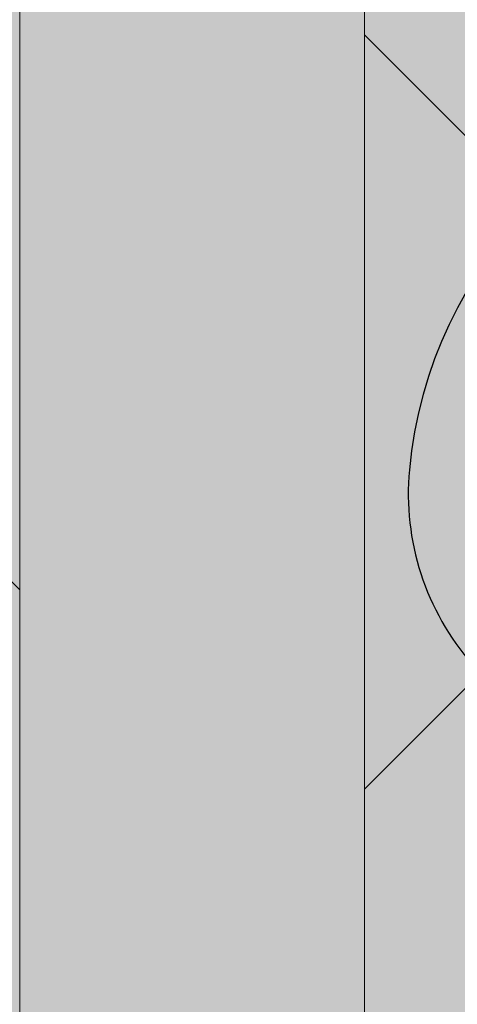
# Model space of a CAD drawing. Units: inches. Extents: x 844 to 2234, y 346 to 1084.
# Tile 17 of 93: x 1117.756 to 1118.565, y 703.242 to 705.06. Entities that reach past the tile are written whole.
import ezdxf

# ---------------------------------------------------------------- set-up
doc = ezdxf.new("R2010")
doc.units = ezdxf.units.IN
doc.header["$MEASUREMENT"] = 0
for name, color, linetype, lineweight in [('A-ANNO-DIMS', 2, 'Continuous', 18), ('furniture', 8, 'Continuous', 18), ('RA-AP-01$0$INT', 35, 'Continuous', 5)]:
    doc.layers.add(name, color=color, linetype=linetype, lineweight=lineweight)
doc.layers.add('RA-AP-01$0$FURN', color=3, linetype='Continuous')
doc.layers.add('RA-AP-01$0$WOOD', color=64, linetype='Continuous')
doc.styles.get("Standard").update_dxf_attribs({"font": 'arial.ttf'})
doc.dimstyles.get("Standard").update_dxf_attribs({"dimtxt": 6, "dimasz": 3, "dimexe": 0.18, "dimexo": 0.0625, "dimgap": 0.09, "dimtad": 0, "dimtih": 1, "dimtoh": 1, "dimdec": 1, "dimzin": 0, "dimdsep": 46, "dimlunit": 3, "dimtxsty": 'Standard', "dimblk": 'ARCHTICK', "dimcen": 0.09, "dimadec": 0, "dimazin": 0, "dimtfac": 1, "dimtdec": 1, "dimtofl": 0, "dimtmove": 0, "dimatfit": 3, "dimfxl": 1, "dimtolj": 1, "dimtzin": 0, "dimarcsym": 0})

# ---------------------------------------------------------------- blocks, each defined once
blk = doc.blocks.new('A$C18D01794')
at = {"layer": 'RA-AP-01$0$INT'}
h = blk.add_hatch(color=256, dxfattribs=at)
h.paths.add_polyline_path([(4.505206456958071, -7.585498806127123), (4.46934859260189, -7.549640941759413), (4.505206456958071, -7.513783077414768), (4.505206456958071, -7.381963272220687), (4.469348592616735, -7.346105407867824), (4.505206456958071, -7.310247543514964), (4.505206456958071, -7.178427738324996), (4.469348592586679, -7.142569873965138), (4.505206456952245, -7.106712009588038), (4.476922185709333, -7.106712009588038), (4.455206456960671, -7.128427738343681), (4.433490728198047, -7.106712009588038), (4.405206456946033, -7.106712009588036), (4.441064321339216, -7.142569873969684), (4.40520645695807, -7.178427738362358), (4.405206456958072, -7.310247543472698), (4.441064321364728, -7.346105407867826), (4.40520645695807, -7.381963272262947), (4.40520645695807, -7.513783077378263), (4.441064321354429, -7.549640941786153), (4.405206456958072, -7.585498806170974), (4.405206456958072, -7.717318611286652), (4.441064321333084, -7.753176475673194), (4.405206456958072, -7.789034340036673), (4.405206456958072, -8.006712009588039), (4.644348592588106, -8.006712009588039), (4.680206456964639, -7.970854145211967), (4.716064321341165, -8.006712009588039), (4.869348592586113, -8.006712009588039), (4.905206456964143, -7.970854145210465), (4.941064321342174, -8.006712009588039), (5.094348592587118, -8.006712009588037), (5.130206456963649, -7.970854145211967), (5.166064321340178, -8.006712009588039), (5.405206456958072, -8.006712009588039), (5.405206456958072, -7.789034340024526), (5.369348592595202, -7.753176475673196), (5.40520645695807, -7.717318611298797), (5.40520645695807, -7.585498806158829), (5.369348592573859, -7.549640941786151), (5.40520645695807, -7.51378307739041), (5.40520645695807, -7.381963272250803), (5.36934859256356, -7.346105407867824), (5.405206456958072, -7.310247543484846), (5.405206456958072, -7.178427738350217), (5.369348592589068, -7.142569873969682), (5.405206456982249, -7.106712009588038), (5.376922185730244, -7.106712009588038), (5.355206456967613, -7.128427738343679), (5.333490728218955, -7.10671200958804), (5.305206456976043, -7.106712009588042), (5.341064321341609, -7.142569873965136), (5.305206456958072, -7.178427738337141), (5.305206456958072, -7.310247543502816), (5.34106432131155, -7.346105407867824), (5.305206456958072, -7.381963272232832), (5.30520645695807, -7.513783077402624), (5.341064321326395, -7.549640941759413), (5.305206456958072, -7.585498806139263), (5.305206456958072, -7.717318611299605), (5.341064321347738, -7.753176475677737), (5.305206456958072, -7.78903434007894), (5.30520645695807, -7.906712009588039), (5.166064321336834, -7.906712009588039), (5.130206456963647, -7.942569873961684), (5.094348592590464, -7.906712009588039), (4.941064321338827, -7.906712009588041), (4.905206456964145, -7.942569873963183), (4.869348592589459, -7.906712009588039), (4.716064321337822, -7.906712009588041), (4.680206456964641, -7.942569873961684), (4.644348592591453, -7.906712009588039), (4.505206456958071, -7.906712009588039), (4.505206456958071, -7.789034340066795), (4.469348592580545, -7.753176475677738), (4.505206456958071, -7.717318611311748)])
h.paths.add_polyline_path([(4.485206456974132, -7.709034340046354), (4.45520645695909, -7.739034340051736), (4.425206456974128, -7.709034340057131), (4.425206456993394, -7.593783077384998), (4.45520645699153, -7.563783077396511), (4.485206456993396, -7.593783077408017)], flags=16)
h.paths.add_polyline_path([(4.455206456954537, -7.767318611299197), (4.485206456958242, -7.797318611312542), (4.48520645695951, -7.912569873958716), (4.45520645695415, -7.942569873954422), (4.425206456957888, -7.912569873967813), (4.425206456957888, -7.797318611286197)], flags=16)
h.paths.add_polyline_path([(4.455206456964794, -7.535498806149051), (4.42520645696469, -7.5054988061393), (4.425206456983954, -7.390247543486406), (4.455206456990734, -7.360247543489279), (4.485206456983953, -7.39024754349214), (4.485206456964687, -7.505498806158811)], flags=16)
h.paths.add_polyline_path([(4.499348592588947, -7.926712009585049), (4.636064321340932, -7.926712009585049), (4.666064321342317, -7.956712009586821), (4.636064321343707, -7.986712009585048), (4.499348592575121, -7.986712009585048), (4.469348592591685, -7.956712009591957)], flags=16)
h.paths.add_polyline_path([(4.425206456957888, -7.940854145195974), (4.471064321332215, -7.986712009585049), (4.425206456957888, -7.986712009585049)], flags=16)
h.paths.add_polyline_path([(4.455206456990734, -7.331963272246367), (4.425206456989053, -7.301963272254337), (4.425206456969784, -7.186712009596224), (4.455206456965226, -7.156712009591144), (4.485206456969787, -7.186712009586051), (4.485206456989053, -7.301963272238404)], flags=16)
h.paths.add_polyline_path([(4.72434859258714, -7.926712009586255), (4.861064321340141, -7.926712009586248), (4.891064321340324, -7.956712009586823), (4.861064321340513, -7.986712009586252), (4.724348592586768, -7.986712009586252), (4.694348592586956, -7.956712009586821)], flags=16)
h.paths.add_polyline_path([(4.919348592587961, -7.956712009586821), (4.949348592588145, -7.92671200958625), (5.08606432134115, -7.926712009586253), (5.116064321341327, -7.956712009586823), (5.086064321341519, -7.986712009586252), (4.949348592587774, -7.986712009586252)], flags=16)
h.paths.add_polyline_path([(5.144348592585967, -7.956712009586823), (5.174348592587358, -7.926712009585049), (5.311064321339338, -7.926712009585049), (5.3410643213366, -7.956712009591957), (5.311064321353163, -7.986712009585048), (5.174348592584576, -7.986712009585048)], flags=16)
h.paths.add_polyline_path([(5.32520645693489, -7.593783077408021), (5.355206456936755, -7.563783077396511), (5.385206456934894, -7.593783077384998), (5.38520645695416, -7.709034340057128), (5.355206456969194, -7.739034340051736), (5.325206456954153, -7.709034340046352)], flags=16)
h.paths.add_polyline_path([(5.325206456970042, -7.797318611312542), (5.355206456973747, -7.767318611299197), (5.385206456970398, -7.7973186112862), (5.385206456970398, -7.912569873967816), (5.355206456974136, -7.942569873954422), (5.325206456968778, -7.912569873958716)], flags=16)
h.paths.add_polyline_path([(5.325206456963599, -7.505498806158811), (5.325206456944333, -7.39024754349214), (5.355206456937552, -7.360247543489279), (5.385206456944332, -7.39024754348641), (5.385206456963596, -7.505498806139303), (5.355206456963492, -7.53549880614905)], flags=16)
h.paths.add_polyline_path([(5.32520645693923, -7.301963272238403), (5.3252064569585, -7.186712009586051), (5.355206456963062, -7.156712009591142), (5.3852064569585, -7.186712009596224), (5.385206456939234, -7.301963272254338), (5.355206456937552, -7.331963272246369)], flags=16)
h.paths.add_polyline_path([(5.339348592596071, -7.986712009585048), (5.385206456970398, -7.940854145195972), (5.385206456970396, -7.986712009585048)], flags=16)
h = blk.add_hatch(color=256, dxfattribs=at)
h.paths.add_polyline_path([(4.469348592586677, -7.142569873965136), (4.505206456958073, -7.178427738324996), (4.505206456958071, -7.106712009582215)])
h.paths.add_polyline_path([(4.455206456960671, -7.128427738343681), (4.476922185709333, -7.106712009588038), (4.433490728198045, -7.106712009588038)])
h.paths.add_polyline_path([(4.405206456958073, -7.178427738362358), (4.441064321339218, -7.142569873969684), (4.40520645695807, -7.106712009600073)])
h.paths.add_polyline_path([(4.425206456989053, -7.301963272254335), (4.455206456990736, -7.331963272246371), (4.485206456989055, -7.301963272238399), (4.48520645696979, -7.186712009586054), (4.455206456965227, -7.15671200959114), (4.425206456969784, -7.186712009596224)])
h.paths.add_polyline_path([(4.505206456958073, -7.381963272220689), (4.505206456958071, -7.310247543514961), (4.469348592616738, -7.346105407867826)])
h.paths.add_polyline_path([(4.425206456964688, -7.5054988061393), (4.455206456964794, -7.535498806149051), (4.485206456964689, -7.505498806158811), (4.485206456983951, -7.390247543492138), (4.455206456990736, -7.360247543489277), (4.425206456983956, -7.39024754348641)])
h.paths.add_polyline_path([(4.425206456974126, -7.709034340057128), (4.455206456959092, -7.739034340051736), (4.485206456974132, -7.709034340046356), (4.485206456993396, -7.593783077408017), (4.45520645699153, -7.563783077396511), (4.425206456993394, -7.593783077384999)])
h.paths.add_polyline_path([(4.46934859260189, -7.549640941759415), (4.505206456958071, -7.585498806127123), (4.505206456958073, -7.513783077414766)])
h.paths.add_polyline_path([(4.405206456958073, -7.585498806170972), (4.441064321354427, -7.549640941786151), (4.405206456958072, -7.513783077378263)])
h.paths.add_polyline_path([(4.405206456958072, -7.789034340036673), (4.441064321333084, -7.753176475673194), (4.405206456958072, -7.71731861128665)])
h.paths.add_polyline_path([(4.469348592580547, -7.75317647567774), (4.505206456958071, -7.789034340066795), (4.505206456958071, -7.717318611311744)])
h.paths.add_polyline_path([(4.425206456957888, -7.912569873967814), (4.45520645695415, -7.942569873954422), (4.485206456959507, -7.912569873958718), (4.48520645695824, -7.797318611312542), (4.455206456954537, -7.767318611299197), (4.425206456957888, -7.797318611286202)])
h.paths.add_polyline_path([(4.425206456957888, -7.986712009585049), (4.471064321332215, -7.986712009585049), (4.425206456957888, -7.940854145195972)])
h.paths.add_polyline_path([(4.499348592575121, -7.986712009585048), (4.636064321343707, -7.986712009585049), (4.666064321342317, -7.956712009586823), (4.636064321340932, -7.926712009585049), (4.499348592588945, -7.926712009585049), (4.469348592591685, -7.95671200959196)])
h.paths.add_polyline_path([(4.680206456964641, -7.942569873961684), (4.716064321337824, -7.906712009588039), (4.644348592591454, -7.906712009588039)])
h.paths.add_polyline_path([(4.644348592588108, -8.006712009588039), (4.716064321341167, -8.006712009588039), (4.680206456964637, -7.970854145211964)])
h.paths.add_polyline_path([(4.724348592586768, -7.98671200958625), (4.861064321340514, -7.986712009586252), (4.891064321340324, -7.956712009586819), (4.861064321340141, -7.92671200958625), (4.724348592587134, -7.926712009586255), (4.694348592586957, -7.956712009586821)])
h.paths.add_polyline_path([(4.905206456964143, -7.942569873963183), (4.941064321338827, -7.906712009588039), (4.869348592589457, -7.906712009588037)])
h.paths.add_polyline_path([(4.869348592586113, -8.006712009588039), (4.941064321342172, -8.006712009588037), (4.905206456964145, -7.970854145210463)])
h.paths.add_polyline_path([(4.949348592587774, -7.986712009586252), (5.086064321341521, -7.986712009586252), (5.116064321341329, -7.956712009586823), (5.08606432134115, -7.926712009586253), (4.949348592588145, -7.92671200958625), (4.919348592587961, -7.956712009586819)])
h.paths.add_polyline_path([(5.130206456963645, -7.942569873961684), (5.166064321336834, -7.906712009588039), (5.094348592590464, -7.906712009588039)])
h.paths.add_polyline_path([(5.094348592587119, -8.006712009588039), (5.166064321340178, -8.006712009588039), (5.130206456963651, -7.970854145211967)])
h.paths.add_polyline_path([(5.174348592584578, -7.986712009585048), (5.311064321353163, -7.986712009585048), (5.341064321336602, -7.956712009591958), (5.31106432133934, -7.926712009585049), (5.174348592587352, -7.926712009585049), (5.144348592585969, -7.956712009586823)])
h.paths.add_polyline_path([(5.325206456968778, -7.912569873958718), (5.355206456974136, -7.942569873954422), (5.385206456970396, -7.912569873967814), (5.385206456970396, -7.797318611286199), (5.355206456973747, -7.767318611299197), (5.325206456970044, -7.797318611312544)])
h.paths.add_polyline_path([(5.339348592596073, -7.986712009585048), (5.385206456970396, -7.986712009585049), (5.385206456970398, -7.94085414519597)])
h.paths.add_polyline_path([(5.325206456954155, -7.709034340046354), (5.355206456969194, -7.739034340051734), (5.38520645695416, -7.709034340057128), (5.385206456934896, -7.593783077384999), (5.355206456936758, -7.563783077396513), (5.325206456934888, -7.593783077408019)])
h.paths.add_polyline_path([(5.305206456958072, -7.789034340078938), (5.341064321347739, -7.753176475677738), (5.305206456958072, -7.717318611299605)])
h.paths.add_polyline_path([(5.369348592595204, -7.753176475673194), (5.40520645695807, -7.789034340024526), (5.405206456958072, -7.717318611298798)])
h.paths.add_polyline_path([(5.405206456958072, -7.585498806158831), (5.405206456958072, -7.513783077390407), (5.369348592573857, -7.549640941786151)])
h.paths.add_polyline_path([(5.305206456958072, -7.585498806139266), (5.341064321326393, -7.549640941759413), (5.305206456958072, -7.513783077402626)])
h.paths.add_polyline_path([(5.325206456963599, -7.50549880615881), (5.355206456963494, -7.535498806149055), (5.385206456963598, -7.505498806139302), (5.385206456944334, -7.390247543486411), (5.355206456937552, -7.360247543489279), (5.325206456944333, -7.39024754349214)])
h.paths.add_polyline_path([(5.305206456958072, -7.38196327223283), (5.341064321311551, -7.346105407867824), (5.305206456958072, -7.31024754350282)])
h.paths.add_polyline_path([(5.325206456939231, -7.301963272238404), (5.355206456937552, -7.331963272246369), (5.385206456939235, -7.301963272254335), (5.385206456958502, -7.186712009596224), (5.355206456963061, -7.156712009591142), (5.3252064569585, -7.186712009586051)])
h.paths.add_polyline_path([(5.404581768715993, -7.381338584008926, -0.001217816984214), (5.405206456958072, -7.381112009582329), (5.405206456958072, -7.310247543484846), (5.369348592563558, -7.346105407867826)])
h.paths.add_polyline_path([(5.36934859258907, -7.142569873969684), (5.40520645695807, -7.178427738350215), (5.405206456958072, -7.106712009612218)])
h.paths.add_polyline_path([(5.355206456967613, -7.128427738343683), (5.376922185730239, -7.106712009588038), (5.333490728218953, -7.10671200958804)])
h.paths.add_polyline_path([(5.30520645695807, -7.178427738337139), (5.341064321341609, -7.142569873965134), (5.305206456958074, -7.10671200957007)])
blk.add_hatch(color=256, dxfattribs=at).paths.add_polyline_path([(4.505206456958071, -7.906712009588039), (5.305206456958072, -7.906712009588039), (5.305206456958072, -7.106712009588038), (5.255206456951893, -7.106712009588036), (5.25520645694868, -7.856712009570104), (4.555206456959269, -7.856712009588616), (4.555206456956052, -7.106712009588038), (4.505206456958073, -7.106712009588038)])
h = blk.add_hatch(color=256, dxfattribs=at)
h.paths.add_polyline_path([(4.585917135068448, -7.856712009587804), (4.614201406330596, -7.856712009587056), (4.668846067270487, -7.802067348644738), (4.723490728212344, -7.856712009584164), (4.771774999457151, -7.856712009582887), (4.826419660396886, -7.80206734864072), (4.862780050090322, -7.838427738332541), (4.844495778842715, -7.856712009580965), (4.862780050090411, -7.856712009580482), (4.905206456960182, -7.814285602707865), (4.947632863832445, -7.856712009578238), (4.965917135079675, -7.856712009577755), (4.947632863831759, -7.838427738330656), (4.983993253523576, -7.802067348637219), (5.038637914464627, -7.856712009575829), (5.08692218571208, -7.856712009574554), (5.141566846649976, -7.802067348634224), (5.196211507589851, -7.856712009571666), (5.224495778822615, -7.856712009570916), (4.905206456953975, -7.537422687702283)])
h.paths.add_polyline_path([(4.895206456956031, -7.575706958950402), (4.895206456958921, -7.684996280828174), (4.840561796018589, -7.630351619890275)], flags=16)
h.paths.add_polyline_path([(4.915206456955638, -7.575706958949956), (4.969851117895509, -7.630351619887399), (4.915206456957609, -7.684996280827732)], flags=16)
h.paths.add_polyline_path([(4.826419660395175, -7.644493755514321), (4.881064321335613, -7.699138416452331), (4.771774999456703, -7.69913841645522)], flags=16)
h.paths.add_polyline_path([(4.983993253519558, -7.644493755510815), (5.038637914460456, -7.699138416449285), (4.929348592581548, -7.69913841645126)], flags=16)
h.paths.add_polyline_path([(4.881064321336025, -7.719138416452334), (4.826419660397532, -7.773783077393256), (4.771774999457062, -7.719138416455217)], flags=16)
h.paths.add_polyline_path([(4.929348592582019, -7.71913841645126), (5.038637914460982, -7.719138416449284), (4.983993253522945, -7.773783077389749)], flags=16)
h.paths.add_polyline_path([(4.895206456960191, -7.733280552075633), (4.895206456962115, -7.806001331460164), (4.876922185715016, -7.824285602708492), (4.840561796021581, -7.787925213016675)], flags=16)
h.paths.add_polyline_path([(4.915206456958487, -7.733280552075187), (4.969851117899527, -7.787925213013798), (4.933490728206909, -7.824285602708034), (4.9152064569598, -7.806001331461736)], flags=16)
h.paths.add_polyline_path([(4.757632863832376, -7.733280552079264), (4.812277524772842, -7.787925213017304), (4.757632863834348, -7.842569873958233)], flags=16)
h.paths.add_polyline_path([(4.737632863832376, -7.73328055207979), (4.737632863834348, -7.842569873958701), (4.682988202893906, -7.787925213020692)], flags=16)
h.paths.add_polyline_path([(5.05278005008503, -7.733280552072701), (5.052780050087917, -7.842569873951664), (4.998135389146995, -7.787925213013169)], flags=16)
h.paths.add_polyline_path([(5.072780050085024, -7.733280552072333), (5.127424711025931, -7.787925213010806), (5.072780050087916, -7.842569873951244)], flags=16)
h.paths.add_polyline_path([(4.935917135072783, -7.506712009583784), (5.255206456948811, -7.826001331459767), (5.255206456948932, -7.797717060211899), (5.200561796010279, -7.743072399273238), (5.255206456949403, -7.688427738334128), (5.25520645694961, -7.640143467086677), (5.200561796009787, -7.585498806146837), (5.236922185702417, -7.549138416454212), (5.255206456949919, -7.56742268770172), (5.255206456949998, -7.549138416454178), (5.212780050078687, -7.506712009583814), (5.25520645695036, -7.464285602712145), (5.255206456950438, -7.446001331464763), (5.236922185702424, -7.464285602712779), (5.200561796009796, -7.427925213020149), (5.255206456950753, -7.373280552079203), (5.25520645695096, -7.324996280834394), (5.200561796010322, -7.270351619893748), (5.255206456951428, -7.215706958952649), (5.255206456951547, -7.187422687705071)])
h.paths.add_polyline_path([(5.042988202883395, -7.42792521302065), (5.097632863823085, -7.373280552080975), (5.097632863822622, -7.482569873959883)], flags=16)
h.paths.add_polyline_path([(5.028846067259663, -7.442067348644384), (5.083490728198774, -7.496712009583504), (4.974201406321001, -7.496712009583035)], flags=16)
h.paths.add_polyline_path([(5.117632863823087, -7.37328055208089), (5.172277524762331, -7.42792521302015), (5.11763286382262, -7.482569873959851)], flags=16)
h.paths.add_polyline_path([(5.08349072819877, -7.516712009582191), (5.028846067259652, -7.571356670521302), (4.974201406320998, -7.516712009582638)], flags=16)
h.paths.add_polyline_path([(5.131774999446817, -7.35913841645716), (5.186419660386065, -7.413783077396415), (5.241064321325782, -7.359138416456712)], flags=17)
h.paths.add_polyline_path([(5.131774999446228, -7.496712009583703), (5.186419660386065, -7.442067348643883), (5.222780050079488, -7.478427738337313), (5.204495778832781, -7.496712009584014)], flags=16)
h.paths.add_polyline_path([(5.097632863822613, -7.530854145205813), (5.097632863823061, -7.640143467084723), (5.042988202883383, -7.585498806145032)], flags=16)
h.paths.add_polyline_path([(5.131774999446899, -7.339138416457162), (5.241064321325809, -7.339138416456712), (5.186419660386591, -7.284493755517479)], flags=17)
h.paths.add_polyline_path([(5.131774999446226, -7.516712009581999), (5.204495778830767, -7.516712009581702), (5.22278005007868, -7.534996280829206), (5.186419660386049, -7.571356670521828)], flags=16)
h.paths.add_polyline_path([(5.11763286382262, -7.530854145205852), (5.17227752476232, -7.585498806145562), (5.117632863823064, -7.64014346708481)], flags=16)
h.paths.add_polyline_path([(5.186419660386069, -7.599640941770585), (5.241064321325754, -7.654285602710281), (5.131774999446791, -7.654285602709814)], flags=16)
h.paths.add_polyline_path([(5.131774999446872, -7.674285602709813), (5.24106432132578, -7.674285602710282), (5.186419660386554, -7.728930263649504)], flags=16)
h.paths.add_polyline_path([(5.255206456951811, -7.126001331467467), (5.255206456951895, -7.106712009588038), (4.555206456956052, -7.106712009588038), (4.555206456956136, -7.12600133146746), (4.905206456953973, -7.476001331465289)])
h.paths.add_polyline_path([(4.983993253513404, -7.368930263651977), (4.92934859257295, -7.314285602713969), (5.03863791445186, -7.314285602711063)], flags=16)
h.paths.add_polyline_path([(4.969851117889988, -7.383072399276016), (4.915206456952556, -7.437717060215906), (4.915206456949648, -7.328427738338133)], flags=16)
h.paths.add_polyline_path([(4.929348592572535, -7.294285602713971), (4.983993253511019, -7.239640941773039), (5.038637914451496, -7.294285602711065)], flags=16)
h.paths.add_polyline_path([(5.052780050074912, -7.280143467087016), (4.998135389134438, -7.225498806148989), (5.052780050072919, -7.170854145208052)], flags=16)
h.paths.add_polyline_path([(5.07278005007491, -7.280143467086489), (5.072780050072918, -7.170854145207579), (5.127424711013374, -7.225498806145578)], flags=16)
h.paths.add_polyline_path([(4.89520645695295, -7.437717060216355), (4.840561796013067, -7.383072399278919), (4.895206456950961, -7.328427738338582)], flags=16)
h.paths.add_polyline_path([(4.915206456948365, -7.280143467090674), (4.915206456946434, -7.207422687704125), (4.933490728192729, -7.18913841645701), (4.969851117886972, -7.225498806149623)], flags=16)
h.paths.add_polyline_path([(4.881064321327021, -7.314285602715054), (4.82641966038902, -7.368930263655506), (4.771774999448108, -7.314285602717047)], flags=16)
h.paths.add_polyline_path([(4.895206456950073, -7.280143467091125), (4.840561796009022, -7.225498806152518), (4.876922185700835, -7.18913841645908), (4.895206456948749, -7.207422687706589)], flags=16)
h.paths.add_polyline_path([(4.983993253510392, -7.211356670525576), (4.947632863816944, -7.174996280833758), (4.965917135064043, -7.156712009585847), (5.038637914448995, -7.156712009584522)], flags=16)
h.paths.add_polyline_path([(4.881064321326543, -7.294285602715056), (4.771774999447578, -7.294285602717046), (4.826419660385607, -7.239640941776569)], flags=16)
h.paths.add_polyline_path([(4.905206456946447, -7.19913841645844), (4.862780050074785, -7.156712009587725), (4.947632863816685, -7.156712009586302)], flags=16)
h.paths.add_polyline_path([(5.14156684663679, -7.211356670521528), (5.086922185696452, -7.156712009583639), (5.196211507574223, -7.156712009581651)], flags=16)
h.paths.add_polyline_path([(4.8264196603837, -7.211356670529104), (4.771774999442643, -7.156712009590501), (4.8444957788276, -7.156712009588568), (4.862780050075511, -7.17499628083566)], flags=16)
h.paths.add_polyline_path([(4.812277524760289, -7.225498806153156), (4.757632863822258, -7.28014346709363), (4.757632863819352, -7.170854145214669)], flags=16)
h.paths.add_polyline_path([(4.73763286382226, -7.280143467093997), (4.682988202881349, -7.22549880615554), (4.737632863819352, -7.170854145215086)], flags=16)
h.paths.add_polyline_path([(4.723490728195188, -7.156712009591787), (4.668846067257299, -7.211356670532127), (4.614201406317417, -7.156712009594693)], flags=16)
h.paths.add_polyline_path([(4.597632863829262, -7.506712009583814), (4.555206456957951, -7.54913841645418), (4.555206456958029, -7.56742268770172), (4.573490728205535, -7.549138416454212), (4.609851117898167, -7.585498806146839), (4.555206456958338, -7.640143467086675), (4.555206456958546, -7.688427738334125), (4.60985111789767, -7.743072399273238), (4.555206456959015, -7.797717060211899), (4.555206456959138, -7.826001331459767), (4.874495778835167, -7.506712009583786), (4.5552064569564, -7.187422687705062), (4.555206456956523, -7.215706958952644), (4.609851117897629, -7.270351619893746), (4.555206456956988, -7.324996280834396), (4.555206456957198, -7.373280552079195), (4.609851117898153, -7.427925213020147), (4.573490728205528, -7.464285602712779), (4.555206456957507, -7.446001331464756), (4.555206456957585, -7.464285602712143)])
h.paths.add_polyline_path([(4.712780050085332, -7.482569873959882), (4.712780050084863, -7.373280552080972), (4.767424711024555, -7.42792521302065)], flags=16)
h.paths.add_polyline_path([(4.726922185709173, -7.496712009583504), (4.781566846648288, -7.442067348644384), (4.836211507586949, -7.496712009583033)], flags=16)
h.paths.add_polyline_path([(4.692780050085327, -7.482569873959851), (4.638135389145619, -7.427925213020149), (4.692780050084865, -7.373280552080892)], flags=16)
h.paths.add_polyline_path([(4.726922185709182, -7.516712009582191), (4.836211507586949, -7.51671200958264), (4.7815668466483, -7.571356670521304)], flags=16)
h.paths.add_polyline_path([(4.678637914461726, -7.496712009583706), (4.605917135075169, -7.496712009584014), (4.587632863828464, -7.478427738337311), (4.623993253521887, -7.442067348643881)], flags=16)
h.paths.add_polyline_path([(4.712780050085336, -7.530854145205816), (4.767424711024568, -7.585498806145034), (4.71278005008489, -7.640143467084724)], flags=16)
h.paths.add_polyline_path([(4.678637914461726, -7.516712009582001), (4.623993253521899, -7.571356670521829), (4.587632863829271, -7.534996280829206), (4.605917135077185, -7.5167120095817)], flags=16)
h.paths.add_polyline_path([(4.692780050085336, -7.530854145205848), (4.692780050084889, -7.64014346708481), (4.638135389145632, -7.585498806145562)], flags=16)
h.paths.add_polyline_path([(4.623993253521885, -7.413783077396415), (4.678637914461131, -7.359138416457161), (4.56934859258217, -7.359138416456712)], flags=17)
h.paths.add_polyline_path([(4.623993253521901, -7.599640941770568), (4.678637914461158, -7.654285602709814), (4.569348592582195, -7.654285602710281)], flags=16)
h.paths.add_polyline_path([(4.678637914461051, -7.339138416457162), (4.623993253521361, -7.284493755517479), (4.569348592582143, -7.339138416456712)], flags=17)
h.paths.add_polyline_path([(4.678637914461076, -7.674285602709813), (4.623993253521399, -7.728930263649504), (4.569348592582167, -7.674285602710281)], flags=16)
h = blk.add_hatch(color=256, dxfattribs=at)
h.paths.add_polyline_path([(4.781566846647504, -7.442067348645805), (4.836211507586161, -7.496712009584463), (4.726922185708388, -7.496712009584918)])
h.paths.add_polyline_path([(4.836211507586161, -7.516712009584068), (4.781566846647504, -7.571356670522723), (4.726922185708388, -7.516712009583606)])
h.paths.add_polyline_path([(4.76742471102377, -7.585498806146453), (4.712780050084083, -7.640143467086137), (4.712780050084542, -7.530854145207227)])
h.paths.add_polyline_path([(4.692780050084544, -7.530854145207257), (4.692780050084084, -7.64014346708622), (4.638135389144834, -7.585498806146965)])
h.paths.add_polyline_path([(4.678637914460932, -7.516712009583407), (4.623993253521102, -7.571356670523233), (4.587632863827676, -7.53499628082981), (4.605917135074382, -7.516712009583104)])
h.paths.add_polyline_path([(4.573490728204743, -7.54913841645434), (4.60985111789737, -7.585498806146969), (4.555206456957541, -7.640143467086797), (4.555206456957237, -7.567422687701846)])
h.paths.add_polyline_path([(4.623993253521098, -7.599640941770699), (4.67863791446035, -7.654285602709951), (4.56934859258139, -7.654285602710407)])
h.paths.add_polyline_path([(4.678637914460275, -7.67428560270995), (4.623993253520583, -7.728930263649637), (4.56934859258136, -7.674285602710405)])
h.paths.add_polyline_path([(4.609851117896854, -7.743072399273369), (4.555206456958196, -7.797717060212026), (4.555206456957738, -7.688427738334254)])
h.paths.add_polyline_path([(4.597632863828475, -7.506712009583301), (4.555206456957283, -7.549138416454495), (4.555206456956805, -7.464285602712587)])
h.paths.add_polyline_path([(4.678637914460932, -7.496712009585113), (4.605917135076396, -7.496712009585417), (4.587632863828479, -7.478427738337913), (4.623993253521104, -7.442067348645284)])
h.paths.add_polyline_path([(4.692780050084091, -7.373280552082301), (4.692780050084548, -7.482569873961267), (4.638135389144834, -7.427925213021552)])
h.paths.add_polyline_path([(4.767424711023772, -7.427925213022072), (4.712780050084545, -7.48256987396129), (4.712780050084089, -7.373280552082384)])
h.paths.add_polyline_path([(4.67863791446036, -7.359138416457298), (4.623993253521105, -7.41378307739655), (4.569348592581399, -7.35913841645684)])
h.paths.add_polyline_path([(4.609851117897371, -7.427925213020278), (4.573490728204743, -7.464285602712907), (4.555206456957237, -7.446001331465401), (4.555206456957548, -7.373280552080448)])
h.paths.add_polyline_path([(4.623993253520596, -7.284493755517612), (4.67863791446028, -7.339138416457299), (4.569348592581367, -7.339138416456838)])
h.paths.add_polyline_path([(4.609851117896867, -7.270351619893878), (4.555206456957749, -7.324996280832994), (4.55520645695821, -7.21570695895522)])
for p, q in [((4.555206456956052, -7.106712009588036), (4.555206456959269, -7.856712009588616)), ((4.555206456958551, -7.68842773833413), (4.60985111789767, -7.743072399273238)), ((4.505206456963013, -7.717318611306806), (4.469348592580547, -7.753176475677738)), ((4.555206456959017, -7.797717060211899), (4.60985111789767, -7.743072399273238))]:
    blk.add_line(p, q, dxfattribs=at)
blk.add_lwpolyline([(5.305206456958072, -7.106712009588038), (5.305206456958072, -7.906712009588039), (4.505206456958071, -7.906712009588039), (4.505206456958071, -7.106712009588038)], dxfattribs=at)
blk = doc.blocks.new('A$C32926AE1')
at = {"layer": 'RA-AP-01$0$WOOD'}
h = blk.add_hatch(color=256, dxfattribs=at)
h.dxf.hatch_style = 1
h.paths.add_polyline_path([(5.157430609644524, 4.573483066760929, -0.1009492694046607), (5.155401577623758, 4.593365984175333, -0.1842662638101597), (5.172249623284174, 4.638795604568598, 0.2056608120311276), (5.179560981299304, 4.661316324430096, 0.3614336704623542), (5.134352340494423, 4.706524965234944, 0.2056608120311297), (5.111831620632933, 4.699213607219793, -0.1842662638101113), (5.066402000239693, 4.682365561559342, -0.1055311479399994), (5.045656153913092, 4.68467289944697, 0.1567636581983829), (4.763886414745334, 4.684672899446966, -0.1055311479399895), (4.743140568418733, 4.68236556155934, -0.1842662638100833), (4.6977109480255, 4.69921360721979, 0.2056608120302612), (4.675190228164109, 4.706524965234949, 0.3614336704708441), (4.629981587358889, 4.66131632442871, 0.2056608120245944), (4.637292945374126, 4.638795604567974, -0.1842662638101024), (4.654140991034615, 4.59336598417475, -0.1009492694055169), (4.652111959013835, 4.573483066760181, 0.021410119221476), (4.629748025606143, 4.156712009541676, 0.0214101192214795), (4.652111959013809, 3.739940952323101, -0.1009492694059586), (4.654140991034615, 3.720058034908448, -0.1842662638100975), (4.637292945374126, 3.674628414515226, 0.2056608120245705), (4.629981587358889, 3.652107694654492, 0.3614336704708879), (4.675190228164113, 3.606899053848249, 0.2056608120302384), (4.697710948025501, 3.614210411863408, -0.1842662638100995), (4.743140568418738, 3.63105845752386, -0.1055311479402541), (4.763886414745388, 3.628751119636215, 0.1567636581983776), (5.045656153913137, 3.628751119636244, -0.1055311479397538), (5.066402000239692, 3.631058457523857, -0.1842662638101067), (5.111831620632931, 3.614210411863407, 0.2056608120310924), (5.134352340494417, 3.606899053848256, 0.3614336704624001), (5.179560981299307, 3.652107694653103, 0.2056608120311314), (5.172249623284175, 3.6746284145146, -0.1842662638101402), (5.155401577623758, 3.72005803490786, -0.1009492694051366), (5.15743060964455, 3.739940952322354, 0.0214101192215073), (5.179794543052287, 4.156712009541468, 0.0214101192215252)])
h.paths.add_polyline_path([(4.639748609479751, 4.156712009541513, 0.0213537860821624), (4.661970494867118, 3.741887061152232, -0.094075836301374), (4.664143710413708, 3.7196126951003, -0.1824818158568985), (4.644813765429836, 3.668037719127816, 0.2056608120245319), (4.639939526753007, 3.653023905887301, 0.3614336704710246), (4.676106439397173, 3.616856993242342, 0.2056608120302234), (4.691120252638095, 3.621731231919122, -0.1824818158602558), (4.742695228611606, 3.641061176902986, -0.1029891339458722), (4.766991894714349, 3.638256818950944, 0.156709409989566), (5.042550673941472, 3.638256818950105, -0.102989133958497), (5.066847340047078, 3.641061176902949, -0.1824818158594995), (5.118422316020358, 3.621731231919103, 0.2056608120311416), (5.133436129261316, 3.616856993242346, 0.3614336704621468), (5.169603041905217, 3.653023905886178, 0.2056608120310986), (5.164728803228477, 3.668037719127177, -0.1824818158565612), (5.145398858244737, 3.719612695099578, -0.0940758363009313), (5.147572073791232, 3.741887061151398, 0.0213537860822023), (5.169793959178681, 4.156712009541451, 0.0213537860822226), (5.147572073791203, 4.571536957931898, -0.0940758363005034), (5.145398858244737, 4.59381132398362, -0.1824818158565587), (5.164728803228476, 4.645386299956021, 0.2056608120311045), (5.169603041905216, 4.66040011319702, 0.3614336704621845), (5.133436129261313, 4.696567025840856, 0.2056608120310773), (5.118422316020359, 4.691692787164098, -0.182481815859508), (5.066847340047078, 4.67236284218025, -0.1029891339584606), (5.04255067394148, 4.675167200133092, 0.156709409989566), (4.766991894714357, 4.675167200132257, -0.1029891339458842), (4.742695228611611, 4.672362842180213, -0.1824818158602725), (4.691120252638095, 4.691692787164077, 0.2056608120302152), (4.676106439397174, 4.696567025840858, 0.3614336704710363), (4.639939526753005, 4.660400113195899, 0.2056608120245495), (4.644813765429837, 4.645386299955384, -0.1824818158568934), (4.664143710413708, 4.593811323982902, -0.0940758363009187), (4.661970494867149, 4.571536957931074, 0.021353786082177)], flags=16)
h.paths.add_polyline_path([(5.129794543052235, 4.432167055276933, -0.0141661062790638), (5.130152669293814, 4.156927903047693, -0.0141661062790647), (5.129794543052234, 3.881688750818433, -0.0785247771143638), (5.10979738006795, 3.755143611847103, 0.0945969212073497), (5.105408519571111, 3.717898134952927, 0.1043170707844957), (5.116074640131521, 3.670385395016088, 0.1043170707864965), (5.068561900193738, 3.681051515576561, 0.09459692119553), (5.031316423304057, 3.676662655080835, -0.1580239521427272), (4.778226145355827, 3.676662655080367, 0.0945969211986668), (4.740980668464973, 3.681051515576592, 0.1043170707882822), (4.693467928526415, 3.670385395015844, 0.1043170707867916), (4.704134049087309, 3.717898134953662, 0.0945969211972894), (4.69974518859162, 3.755143611844042, -0.0785247771163196), (4.679748025606343, 3.881688750818406, -0.0141661062790663), (4.679389899364763, 4.156927903047693, -0.0141661062790672), (4.679748025606343, 4.432167055276998, -0.0785247771163064), (4.699745188591625, 4.55871219425134, 0.094596921197333), (4.704134049087308, 4.595957671141738, 0.1043170707867205), (4.693467928526416, 4.643470411079523, 0.1043170707882628), (4.740980668464965, 4.632804290518776, 0.0945969211988114), (4.778226145355874, 4.637193151015016, -0.158023952142669), (5.031316423304015, 4.637193151014546, 0.0945969211956361), (5.068561900193736, 4.632804290518806, 0.1043170707864979), (5.11607464013152, 4.643470411079278, 0.1043170707844617), (5.105408519571112, 4.595957671142455, 0.0945969212074597), (5.109797380067959, 4.558712194248236, -0.0785247771143467)], flags=0)
h.paths.add_polyline_path([(5.119794532311105, 4.432259799204851, -0.0142000800617244), (5.120156169157484, 4.156927903047701, -0.0142000800617277), (5.119794532311105, 3.881596006890482, -0.0784894509520253), (5.100273383573699, 3.758192358677797, 0.0940138827242913), (5.095413455884425, 3.717477693979438, 0.0606271852308753), (5.099615656341024, 3.686844378806616, 0.0606271852322524), (5.068982341167493, 3.691046579263239, 0.0940138827010453), (5.028267676478798, 3.686186651576848, -0.1580706864508061), (4.781274892180912, 3.686186651576435, 0.0940138827026903), (4.740560227491556, 3.691046579263279, 0.0606271852339895), (4.709926912317155, 3.686844378806508, 0.0606271852329405), (4.714129112773991, 3.717477693980356, 0.094013882701304), (4.709269185087677, 3.758192358669163, -0.0784894509577193), (4.689748036347473, 3.881596006890469, -0.014200080061729), (4.689386399501094, 4.156927903047709, -0.0142000800617217), (4.689748036347473, 4.432259799204808, -0.078489450957724), (4.709269185087651, 4.555663447426125, 0.0940138827014585), (4.714129112773992, 4.596378112114996, 0.0606271852329731), (4.709926912317154, 4.62701142728886, 0.0606271852340196), (4.74056022749157, 4.622809226832087, 0.0940138827024997), (4.781274892180847, 4.627669154518912, -0.1580706864508359), (5.028267676478777, 4.627669154518526, 0.0940138827010946), (5.068982341167492, 4.622809226832129, 0.060627185232254), (5.099615656341024, 4.627011427288751, 0.0606271852308727), (5.095413455884425, 4.59637811211593, 0.0940138827241088), (5.100273383573675, 4.555663447417647, -0.0784894509520978)], flags=0)
h.paths.add_polyline_path([(5.06978912287499, 4.430218106756144, -0.014241683694547), (5.070173729147532, 4.156927903047672, -0.0142416836945458), (5.06978912287499, 3.883637699339223, -0.0800609523125196), (5.052662118612511, 3.773463122773442, 0.0526421978001116), (5.04590916754064, 3.740550867606997, 0.0526421977992423), (5.012996912374707, 3.73379791653534, -0.1583028414718258), (4.796545656286308, 3.73379791653451, 0.0526421978034211), (4.763633401117837, 3.740550867607021, 0.0526421978018622), (4.756880450045755, 3.773463122774558, -0.0800609523117106), (4.739753445783639, 3.883637699339268, -0.0142416836945435), (4.739368839511098, 4.156927903047671, -0.0142416836945477), (4.739753445783639, 4.430218106756155, -0.0800609523116345), (4.75688045004574, 4.540392683320762, 0.052642197801941), (4.763633401117837, 4.573304938488346, 0.0526421978035071), (4.796545656286361, 4.580057889560873, -0.1583028414717561), (5.012996912374669, 4.580057889560039, 0.0526421977993048), (5.04590916754064, 4.57330493848837, 0.0526421978002057), (5.052662118612529, 4.540392683321868, -0.080060952312477)], flags=0)
h.paths.add_polyline_path([(5.049789715110557, 4.43038092723357, -0.0143097550741839), (5.05018085590259, 4.156927903047715, -0.0143097550741854), (5.049789715110558, 3.883474878861827, -0.0800685599149176), (5.03362098255317, 3.779581877367999, 0.0306258898956367), (5.028241146483733, 3.758218888663947, 0.0306258898977031), (5.006878157778253, 3.75283905259408, -0.1583983521624096), (4.802664410878162, 3.752839052594731, 0.0306258898946014), (4.781301422174808, 3.758218888663924, 0.0306258898967912), (4.775921586105202, 3.779581877368794, -0.080068559914251), (4.759752853548071, 3.883474878861786, -0.0143097550741854), (4.759361712756037, 4.156927903047671, -0.0143097550741854), (4.759752853548071, 4.430380927233557, -0.0800685599142479), (4.775921586105193, 4.534273928726546, 0.0306258898968306), (4.781301422174808, 4.555636917431444, 0.0306258898945754), (4.802664410878143, 4.561016753500631, -0.1583983521624168), (5.006878157778244, 4.561016753501291, 0.0306258898977177), (5.028241146483733, 4.555636917431421, 0.0306258898958182), (5.03362098255321, 4.534273928727244, -0.080068559914796)], flags=0)
h.paths.add_polyline_path([(4.999766070382627, 4.428171244713864, -0.0143443147609634), (5.000198441819402, 4.156927903047689, -0.0143443147609612), (4.999766070382627, 3.885684561381556, -0.0784641635803329), (4.987356730658798, 3.799103304488872, -0.1506053783831347), (4.822185837999821, 3.79910330448882, -0.0784641635803318), (4.809776498276007, 3.885684561381509, -0.014344314760963), (4.809344126839227, 4.156927903047677, -0.0143443147609645), (4.809776498276007, 4.428171244713873, -0.0784641635803192), (4.822185837999822, 4.514752501606549, -0.1506053783831338), (4.987356730658798, 4.514752501606494, -0.078464163580285)], flags=0)
h.paths.add_polyline_path([(4.979755254238824, 4.42764379880488, -0.0143772539198268), (4.980205517789977, 4.156927903047693, -0.0143772539198275), (4.979755254238824, 3.886212007290489, -0.0689242507424422), (4.971183264704897, 3.815276770442801, -0.1296645318904179), (4.838359303953726, 3.815276770442746, -0.0689242507424186), (4.829787314419809, 3.886212007290419, -0.0143772539198292), (4.829337050868653, 4.156927903047653, -0.0143772539198325), (4.829787314419809, 4.427643798804946, -0.0689242507424211), (4.838359303953725, 4.498579035652621, -0.1296645318904187), (4.971183264704897, 4.498579035652565, -0.0689242507424401)], flags=0)
for centre, radius, start, end in [((4.679771284329349, 4.656735268264593), 0.0499999999998897, 95.25687599443106, 174.7431240064049), ((4.659855405541232, 4.658567690730234), 0.0300000000000005, 174.7431240062535, 221.2289490796905)]:
    blk.add_arc(centre, radius, start, end, dxfattribs=at)
blk = doc.blocks.new('A$C5D2F253E')
at = {"layer": 'RA-AP-01$0$FURN', "xscale": -0.7999999999883585, "yscale": 0.7999999999883585, "zscale": 0.8, "rotation": 90}
blk.add_blockref('A$C18D01794', (-5.687757199772477, 4.75791982714071), dxfattribs=at)
at = {"layer": 'RA-AP-01$0$WOOD', "rotation": 270}
blk.add_blockref('A$C32926AE1', (-4.161339601644158, 5.73852594588169), dxfattribs=at)
blk = doc.blocks.new('_ArchTick')
at = {"color": 0, "linetype": 'ByBlock', "const_width": 0.15}
blk.add_lwpolyline([(-0.5, -0.5), (0.5, 0.5)], dxfattribs=at)
blk = doc.blocks.new('*D144')
at = {"layer": 'A-ANNO-DIMS', "color": 0, "lineweight": -2, "transparency": 16777216}
for p, q in [((1096.615948, 439.3732739999999), (1096.615948, 1074.743301)), ((1143.115948, 492.373274), (1143.115948, 1074.743301)), ((1096.615948, 1074.563301), (1102.481950728513, 1074.563301)), ((1143.115948, 1074.563301), (1137.249945271487, 1074.563301))]:
    blk.add_line(p, q, dxfattribs=at)
at = {"layer": 'Defpoints', "color": 0, "transparency": 16777216}
for p in [(1143.115948, 1074.563301), (1143.115948, 492.3107739999999), (1096.615948, 439.3107739999999)]:
    blk.add_point(p, dxfattribs=at)
at = {"layer": 'A-ANNO-DIMS', "color": 0, "lineweight": -2, "transparency": 16777216, "xscale": 3, "yscale": 3, "zscale": 3, "rotation": 180}
blk.add_blockref('_ArchTick', (1096.615948, 1074.563301), dxfattribs=at)
at = {"layer": 'A-ANNO-DIMS', "color": 0, "lineweight": -2, "transparency": 16777216, "xscale": 3, "yscale": 3, "zscale": 3}
blk.add_blockref('_ArchTick', (1143.115948, 1074.563301), dxfattribs=at)
at = {"layer": 'A-ANNO-DIMS', "color": 0, "transparency": 16777216, "insert": (1119.865948, 1074.563301), "char_height": 6, "attachment_point": 5}
blk.add_mtext('\\A1;3\'-10 1/2"', dxfattribs=at)

msp = doc.modelspace()

# ---------------------------------------------------------------- block references
at = {"layer": 'furniture', "xscale": 15.94108302203742, "yscale": 15.94108302203742, "zscale": 15.94108302203742, "rotation": 90}
msp.add_blockref('A$C5D2F253E', (1136.147844094663, 696.2584716700112), dxfattribs=at)

# ---------------------------------------------------------------- dimensions: what is measured, and where the dimension line sits
at = {"layer": 'A-ANNO-DIMS'}
dim = msp.add_linear_dim(base=(1143.115948, 1074.563301), p1=(1096.615948, 439.3107739999999), p2=(1143.115948, 492.3107739999999), dimstyle='Standard', override={"dimdec": 1, "dimlfac": 1, "dimrnd": 0, "dimzin": 1, "dimdsep": 46, "dimlunit": 4, "dimfrac": 2}, dxfattribs=at)
dim.commit()
dim.dimension.update_dxf_attribs({"geometry": '*D144', "text_midpoint": (1119.865948, 1074.563301)})

doc.saveas('drawing.dxf')
